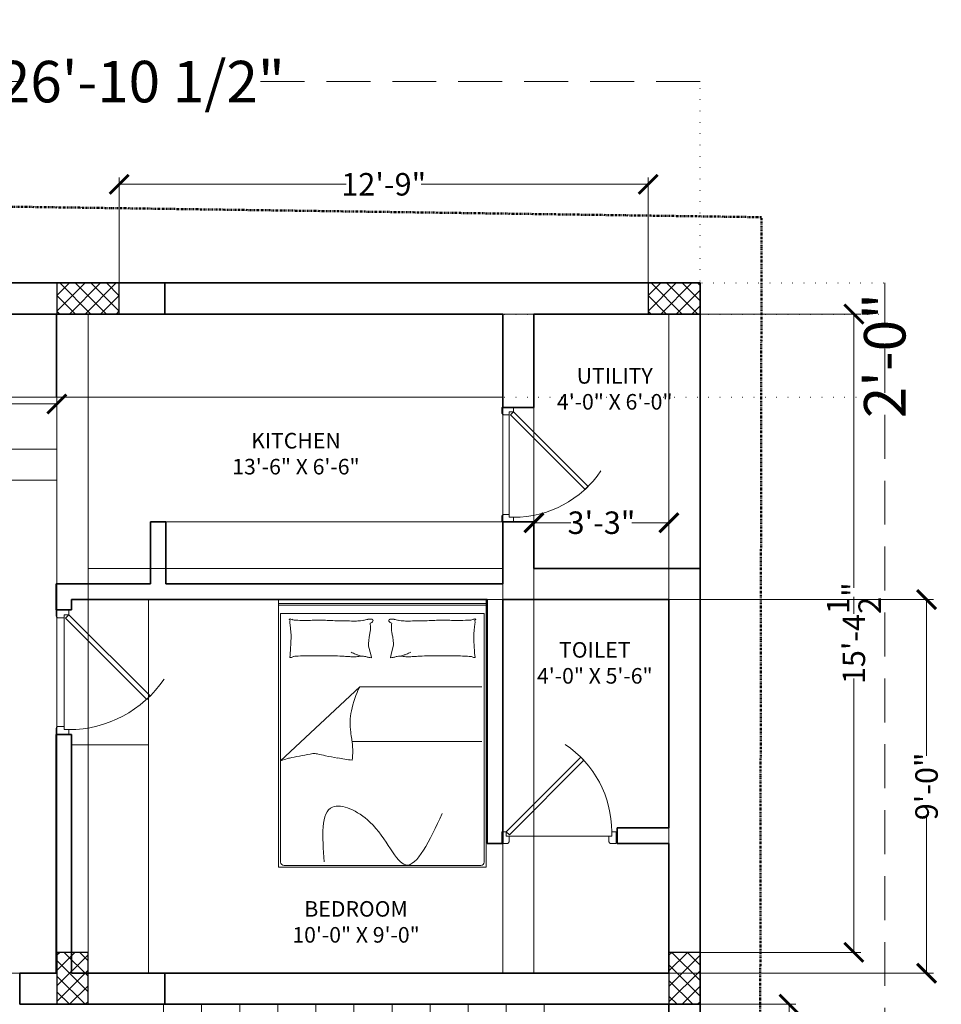
# Model space of a CAD drawing. Units: inches. Extents: x -16911 to -9621, y -48626 to -46270.
# Tile 14 of 20: x -11935 to -11669, y -46595 to -46311. Entities that reach past the tile are written whole.
import ezdxf

# ---------------------------------------------------------------- set-up
doc = ezdxf.new("R2010")
doc.units = ezdxf.units.IN
for name, pattern in [('DASHDOT', [1, 0.5, -0.25, 0, -0.25]), ('DASHED', [19.05, 12.7, -6.35]), ('DOT2', [3.175, 0, -3.175])]:
    doc.linetypes.add(name, pattern=pattern)
for name, color, linetype, lineweight in [('A-ANNO-DIMS', 2, 'Continuous', 13), ('A-AREA-IDEN', 3, 'Continuous', 18), ('A-DOOR', 4, 'Continuous', 18), ('A-FLOR-STRS', 3, 'Continuous', 18), ('A-FURN', 8, 'Continuous', 13), ('A-WALL', 7, 'Continuous', 35), ('C-PROP', 6, 'DASHDOT', 50), ('column', 12, 'Continuous', 30), ('DOOR', 143, 'Continuous', 9), ('EXT BEAM', 132, 'Continuous', 13), ('furniture', 35, 'Continuous', 15), ('S-BEAM', 132, 'Continuous', 25), ('S-COLS', 1, 'Continuous', 30)]:
    doc.layers.add(name, color=color, linetype=linetype, lineweight=lineweight)
doc.styles.add('style3', font='times.ttf')
doc.styles.add('style9', font='swisscl.ttf', dxfattribs={"height": 12})
doc.dimstyles.new('Dim9', dxfattribs={"dimtxt": 10, "dimasz": 0.199219, "dimexe": 1, "dimexo": 0.5, "dimgap": 1, "dimtad": 0, "dimdec": 1, "dimzin": 0, "dimdsep": 46, "dimlunit": 4, "dimtxsty": 'style9', "dimblk": 'ARCHTICK', "dimcen": 0.09, "dimclrd": 256, "dimclrt": 256, "dimadec": 0, "dimazin": 0, "dimtfac": 1, "dimtdec": 1, "dimtix": 1, "dimtofl": 0, "dimtmove": 1, "dimatfit": 3, "dimfxl": 9, "dimtolj": 1, "dimtzin": 0, "dimlwd": -1, "dimarcsym": 0})
doc.dimstyles.new('S.S.S', dxfattribs={"dimtxt": 6.5, "dimasz": 5.5, "dimexe": 2, "dimexo": 0, "dimgap": 0.09, "dimtad": 0, "dimdec": 1, "dimzin": 3, "dimdsep": 46, "dimlunit": 4, "dimtxsty": 'style3', "dimblk": 'ARCHTICK', "dimcen": 2.5, "dimclrd": 252, "dimclre": 256, "dimclrt": 7, "dimadec": 0, "dimazin": 0, "dimtfac": 1, "dimtdec": 1, "dimtix": 1, "dimtofl": 0, "dimtmove": 0, "dimatfit": 3, "dimfxl": 2, "dimtolj": 1, "dimtzin": 0, "dimlwd": 13, "dimlwe": 15, "dimarcsym": 0})

# ---------------------------------------------------------------- blocks, each defined once
blk = doc.blocks.new('hjuyuiuyk')
at = {"layer": 'furniture'}
for p, q in [((-19327.49, -39738.98), (-19327.49, -39737.31)), ((-19327.49, -39737.31), (-19267.49, -39737.31, 0)), ((-19327.49, -39746.54), (-19327.49, -39737.31)), ((-19267.49, -39738.5), (-19327.49, -39738.5, 0)), ((-19327.49, -39738.5, 0), (-19327.49, -39814.72, 0)), ((-19327.49, -39738.5), (-19327.49, -39814.72)), ((-19267.49, -39738.5, 0), (-19327.49, -39738.5)), ((-19267.49, -39738.98, 0), (-19327.49, -39738.98)), ((-19267.49, -39737.31, 0), (-19267.49, -39738.98, 0)), ((-19267.49, -39746.54, 0), (-19267.49, -39737.31, 0)), ((-19267.49, -39814.72), (-19267.49, -39738.5)), ((-19267.49, -39814.72, 0), (-19267.49, -39738.5, 0)), ((-19268.1, -39741.33), (-19326.9, -39741.33)), ((-19326.9, -39741.33), (-19326.9, -39813.21)), ((-19268.1, -39813.21), (-19268.1, -39741.33)), ((-19300.88, -39753.22, 0), (-19301.49, -39750.81, 0)), ((-19294.97, -39753.22, 0), (-19294.37, -39750.81, 0)), ((-19300.67, -39754.09, 0), (-19300.88, -39753.22, 0)), ((-19295.19, -39754.09, 0), (-19294.97, -39753.22, 0)), ((-19304.07, -39762.52), (-19326.9, -39783.91)), ((-19304.07, -39762.52), (-19268.82, -39762.52)), ((-19268.82, -39778.34), (-19306.29, -39778.34)), ((-19326.9, -39813.21), (-19326.9, -39783.91)), ((-19327.49, -39814.72, 0), (-19267.49, -39814.72)), ((-19327.49, -39814.72), (-19267.49, -39814.72, 0)), ((-19269.1, -39814.21), (-19325.9, -39814.21)), ((-19325.9, -39814.21), (-19269.1, -39814.21))]:
    blk.add_line(p, q, dxfattribs=at)
for centre, radius, start, end in [((-19324.36, -39743.07, 0), 0.0997, 111.7883, 160.436), ((-19324.39, -39743.06, 0), 0.0676, 160.436, 281.8931), ((-19324.12, -39743.66, 0), 0.732, 94.3025, 111.7883), ((-19324.35, -39743.25, 0), 0.125, 21.9904, 101.8931), ((-19323.34, -39743.89, 0), 0.956, 158.579, 188.1335), ((-19317.18, -39743.01, 0), 7.17, 188.1335, 192.1095), ((-19324.65, -39743.37, 0), 0.455, 338.579, 21.9904), ((-19329.85, -39745.73, 0), 5.78, 7.6809, 12.1095), ((-19324.11, -39743.77, 0), 0.842, 59.3487, 94.3025), ((-19350.51, -39748.51, 0), 26.62, 3.3687, 7.6809), ((-19322.88, -39741.69, 0), 1.57, 239.3487, 264.7408), ((-19319.6, -39692.5, 0), 50.87, 266.1399, 268.6002), ((-19319.84, -39713.09, 0), 30.28, 268.0921, 271.2808), ((-19320.24, -39695.07, 0), 48.31, 271.2808, 273.4034), ((-19316.15, -39763.89, 0), 20.63, 90.1553, 93.4034), ((-19316.09, -39783.15, 0), 39.89, 86.9902, 90.1553), ((-19305.86, -39588.51, 0), 155.02, 266.9902, 268.5957), ((-19305.42, -39570.46, 0), 173.07, 268.5957, 270), ((-19305.42, -39718.38, 0), 25.15, 270, 273.6841), ((-19304.03, -39739.9, 0), 3.58, 273.6841, 287.1951), ((-19300.46, -39751.46, 0), 8.51, 98.4372, 107.1951), ((-19301.02, -39747.69, 0), 4.7, 90, 98.4372), ((-19301.12, -39743.14, 0), 0.997, 274.4002, 333.4195), ((-19315.3, -39745.68, 0), 14.34, 360, 6.2324), ((-19306.91, -39745.68, 0), 5.95, 350.3156, 360), ((-19301.02, -39745.63, 0), 2.64, 78.7276, 90), ((-19300.58, -39743.42, 0), 0.383, 333.4195, 78.7276), ((-19295.28, -39743.42, 0), 0.383, 101.2724, 206.5805), ((-19294.73, -39743.14, 0), 0.997, 206.5805, 265.5998), ((-19294.84, -39745.63, 0), 2.64, 90, 101.2724), ((-19280.55, -39745.68, 0), 14.34, 173.7676, 180), ((-19288.94, -39745.68, 0), 5.95, 180, 189.6844), ((-19294.84, -39747.69, 0), 4.7, 81.5628, 90), ((-19295.39, -39751.46, 0), 8.51, 72.8049, 81.5628), ((-19291.82, -39739.9, 0), 3.58, 252.8049, 266.3159), ((-19290.43, -39718.38, 0), 25.15, 266.3159, 270), ((-19290.43, -39570.46, 0), 173.07, 270, 271.4043), ((-19289.99, -39588.51, 0), 155.02, 271.4043, 273.0098), ((-19279.76, -39783.15, 0), 39.89, 89.8447, 93.0098), ((-19279.7, -39763.89, 0), 20.63, 86.5966, 89.8447), ((-19275.61, -39695.07, 0), 48.31, 266.5966, 268.7192), ((-19276.02, -39713.09, 0), 30.28, 268.7192, 271.9079), ((-19276.73, -39645.13, 0), 98.25, 271.0069, 272.7772), ((-19272.12, -39741.69, 0), 1.57, 275.2592, 300.6513), ((-19270.89, -39743.77, 0), 0.842, 85.6975, 120.6513), ((-19244.49, -39748.51, 0), 26.62, 172.3191, 176.6313), ((-19265.15, -39745.73, 0), 5.78, 167.8905, 172.3191), ((-19270.88, -39743.66, 0), 0.732, 68.2117, 85.6975), ((-19270.35, -39743.37, 0), 0.455, 158.0096, 201.421), ((-19277.82, -39743.01, 0), 7.17, 347.8905, 351.8665), ((-19270.65, -39743.25, 0), 0.125, 78.1069, 158.0096), ((-19271.66, -39743.89, 0), 0.956, 351.8665, 21.421), ((-19270.61, -39743.06, 0), 0.0676, 258.1069, 19.564), ((-19270.64, -39743.07, 0), 0.0997, 19.564, 68.2117), ((-19343.69, -39748.11, 0), 19.79, 358.3669, 3.3687), ((-19282.35, -39751.13, 0), 19.21, 171.9949, 177.3351), ((-19292.22, -39749.75, 0), 9.25, 167.8016, 171.9949), ((-19326.4, -39742.36, 0), 25.72, 347.8016, 350.3156), ((-19269.45, -39742.36, 0), 25.72, 189.6844, 192.1984), ((-19303.63, -39749.75, 0), 9.25, 8.0051, 12.1984), ((-19313.5, -39751.13, 0), 19.21, 2.6649, 8.0051), ((-19251.31, -39748.11, 0), 19.79, 176.6313, 181.6331), ((-19720.99, -39728.47, 0), 397.61, 356.4951, 356.945), ((-19363.7, -39747.54, 0), 39.81, 356.945, 358.3669), ((-19299.57, -39750.33, 0), 1.97, 177.3351, 194.0452), ((-19296.28, -39750.33, 0), 1.97, 345.9548, 2.6649), ((-19231.3, -39747.54, 0), 39.81, 181.6331, 183.055), ((-18874.01, -39728.47, 0), 397.61, 183.055, 183.5049), ((-19323.69, -39753.93, 0), 0.564, 170.0016, 196.6978), ((-19333.47, -39752.21, 0), 9.37, 350.0016, 356.4951), ((-19324.19, -39754.08, 0), 0.0385, 196.6978, 277.1204), ((-19324.51, -39751.59, 0), 2.55, 277.1204, 286.2212), ((-19324.42, -39751.9, 0), 2.23, 286.2212, 297.4439), ((-19322.81, -39754.99, 0), 1.25, 102.448, 117.4439), ((-19322.32, -39757.22, 0), 3.54, 93.574, 102.448), ((-19318.44, -39837.61, 0), 84.03, 90.9755, 92.7955), ((-19315.55, -39952.16, 0), 198.61, 89.4461, 91.2473), ((-19314.9, -39885.06, 0), 131.51, 87.2326, 89.4461), ((-19310.57, -39795.48, 0), 41.81, 85.4012, 87.2326), ((-19304.32, -39717.78, 0), 36.14, 265.4012, 267.3712), ((-19297.32, -39733.09, 0), 21.54, 244.6889, 246.5156), ((-19305.66, -39747.05, 0), 6.83, 267.3712, 281.4827), ((-19297.32, -39733.09, 0), 21.54, 246.5156, 248.3423), ((-19297.32, -39733.09, 0), 21.54, 248.3423, 250.572), ((-19297.32, -39733.09, 0), 21.54, 250.572, 252.8018), ((-19303.46, -39757.91, 0), 4.25, 83.5659, 101.4827), ((-19303.37, -39757.16, 0), 3.49, 72.6136, 83.5659), ((-19300.33, -39747.43, 0), 6.7, 252.6136, 260.5159), ((-19300.13, -39746.25, 0), 7.9, 260.5159, 265.9171), ((-19300.69, -39754.1, 0), 0.0267, 265.9171, 14.0449), ((-19295.16, -39754.1, 0), 0.0267, 165.9551, 274.0829), ((-19295.72, -39746.25, 0), 7.9, 274.0829, 279.4841), ((-19295.52, -39747.43, 0), 6.7, 279.4841, 287.3864), ((-19292.48, -39757.16, 0), 3.49, 96.4341, 107.3864), ((-19292.39, -39757.91, 0), 4.25, 78.5173, 96.4341), ((-19298.54, -39733.09, 0), 21.54, 287.1982, 289.428), ((-19290.19, -39747.05, 0), 6.83, 258.5173, 272.6288), ((-19298.54, -39733.09, 0), 21.54, 289.428, 291.6577), ((-19298.54, -39733.09, 0), 21.54, 291.6577, 293.4844), ((-19298.54, -39733.09, 0), 21.54, 293.4844, 295.3111), ((-19291.53, -39717.78, 0), 36.14, 272.6288, 274.5988), ((-19285.28, -39795.48, 0), 41.81, 92.7674, 94.5988), ((-19280.95, -39885.06, 0), 131.51, 90.5539, 92.7674), ((-19280.3, -39952.16, 0), 198.61, 88.7527, 90.5539), ((-19277.1, -39805.01, 0), 51.42, 86.426, 88.7527), ((-19274.68, -39799.75, 0), 46.07, 86.5575, 89.0171), ((-19272.19, -39754.99, 0), 1.25, 62.5561, 77.552), ((-19270.58, -39751.9, 0), 2.23, 242.5561, 253.7788), ((-19270.49, -39751.59, 0), 2.55, 253.7788, 262.8796), ((-19261.53, -39752.21, 0), 9.37, 183.5049, 189.9984), ((-19270.81, -39754.08, 0), 0.0385, 262.8796, 343.3022), ((-19271.31, -39753.93, 0), 0.564, 343.3022, 9.9984), ((-19279.47, -39774.89), 27.53, 153.3084, 168.7423), ((-19287.94, -39773.2), 18.89, 168.7423, 187.3994), ((-19242.78, -39767.34), 64.43, 187.3994, 189.2719), ((-19333.07, -39782.08), 27.05, 6.3817, 9.2719), ((-19321.79, -39780.82), 15.7, 359.2313, 6.3817), ((-19287.64, -39956.87), 177.57, 99.7243, 101.7196), ((-19317.24, -39783.9), 2.09, 82.2696, 100.7276), ((-19317.9, -39788.76), 6.99, 76.8096, 82.2696), ((-19295.64, -39693.77), 90.57, 256.8096, 258.3259), ((-19295.11, -39691.23), 93.17, 258.3259, 260.505), ((-19336.71, -39780.62), 30.63, 354.1141, 359.2313), ((-19306.77, -39846.83), 66.07, 105.9352, 107.7364), ((-19318.41, -39806.06), 23.67, 102.9255, 105.9352), ((-19288.03, -39648.9), 136.08, 260.505, 262.308), ((-19325.9, -39813.21), 1, 180, 270), ((-19269.1, -39813.21), 1, 270, 0)]:
    blk.add_arc(centre, radius, start, end, dxfattribs=at)
blk.add_open_spline([(-19280.24, -39799.21), (-19283.87, -39806.94), (-19290.73, -39821.55), (-19298.08, -39801.09), (-19315.85, -39793.47), (-19314.86, -39805.92), (-19314.29, -39813.13)], degree=3, knots=[0, 0, 0, 0, 18.167809, 34.338432, 45.972904, 61.997799, 61.997799, 61.997799, 61.997799], dxfattribs=at)
blk = doc.blocks.new('A$C1C9D3E54')
at = {"layer": 'DOOR'}
blk.add_line((18676.53, 5780.72), (18710.53, 5780.72), dxfattribs=at)
blk.add_lwpolyline([(18685.01, 5806.62), (18710.47, 5781.16), (18711.53, 5782.22), (18686.07, 5807.68), (18685.01, 5806.62)], dxfattribs=at)
blk.add_lwpolyline([(18674.03, 5778.22), (18676.03, 5778.22), (18674.03, 5778.22), (18674.03, 5782.22), (18675.53, 5782.22), (18675.53, 5780.72), (18676.53, 5780.72), (18676.53, 5778.72), (18676.41, 5778.72), (18676.41, 5778.6, -0.414214), (18676.16, 5778.35), (18676.03, 5778.35), (18676.03, 5778.22)], format="xyb", dxfattribs=at)
blk.add_lwpolyline([(18713.03, 5782.22), (18711.53, 5782.22), (18711.53, 5780.72), (18710.53, 5780.72), (18710.53, 5778.72), (18710.66, 5778.72), (18710.66, 5778.6, 0.414214), (18710.91, 5778.35), (18711.03, 5778.35), (18711.03, 5778.22), (18713.03, 5778.22), (18711.03, 5778.22), (18713.03, 5778.22), (18713.03, 5782.22)], format="xyb", close=True, dxfattribs=at)
blk.add_arc((18711.53, 5782.22), 36, 124.0336, 180, dxfattribs=at)
blk = doc.blocks.new('COLUMNS')
at = {"layer": 'column'}
h = blk.add_hatch(dxfattribs=at)
h.set_pattern_fill('ANSI37', color=256, angle=-810)
h.set_pattern_definition([(315, (-70004.5392, -80151.7886), (2.24506403, 2.24506403), []), (45, (-70004.5392, -80151.7886), (-2.24506403, 2.24506403), [])])
h.paths.add_polyline_path([(-11924.72, -46386.86), (-11924.72, -46395.86), (-11906.72, -46395.86), (-11906.72, -46386.86)])
h = blk.add_hatch(dxfattribs=at)
h.set_pattern_fill('ANSI37', color=256, angle=-810)
h.set_pattern_definition([(315, (-69833.7395, -80151.7886), (2.24506403, 2.24506403), []), (45, (-69833.7395, -80151.7886), (-2.24506403, 2.24506403), [])])
h.paths.add_polyline_path([(-11753.92, -46386.86), (-11753.92, -46395.86), (-11738.92, -46395.86), (-11738.92, -46386.86)])
h = blk.add_hatch(dxfattribs=at)
h.set_pattern_fill('ANSI37', color=256, angle=-720)
h.set_pattern_definition([(45, (21840.2088, -104675.1704), (-2.24506403, 2.24506403), []), (135, (21840.2088, -104675.1704), (-2.24506403, -2.24506403), [])])
h.paths.add_polyline_path([(-11924.72, -46595.36), (-11915.72, -46595.36), (-11915.72, -46580.36), (-11924.72, -46580.36)])
h = blk.add_hatch(dxfattribs=at)
h.set_pattern_fill('ANSI37', color=256, angle=-900)
h.set_pattern_definition([(225, (-45503.8578, 11499.4594), (2.24506403, -2.24506403), []), (315, (-45503.8578, 11499.4594), (2.24506403, 2.24506403), [])])
h.paths.add_polyline_path([(-11738.92, -46580.36), (-11747.92, -46580.36), (-11747.92, -46595.36), (-11738.92, -46595.36)])
at = {"layer": 'column', "ltscale": 0.05}
for points in [[(-11906.72, -46395.86), (-11906.72, -46386.86), (-11924.72, -46386.86), (-11924.72, -46395.86)], [(-11738.92, -46395.86), (-11738.92, -46386.86), (-11753.92, -46386.86), (-11753.92, -46395.86)], [(-11915.72, -46580.36), (-11924.72, -46580.36), (-11924.72, -46595.36), (-11915.72, -46595.36)], [(-11747.92, -46595.36), (-11738.92, -46595.36), (-11738.92, -46580.36), (-11747.92, -46580.36)]]:
    blk.add_lwpolyline(points, close=True, dxfattribs=at)
blk = doc.blocks.new('TYPICAL BEAMS G-2')
at = {"layer": 'EXT BEAM'}
for p, q in [((-12061.47, -47658.74), (-11738.92, -47658.74)), ((-11738.92, -48216.7), (-11738.92, -47658.74)), ((-12052.47, -47667.74), (-11924.72, -47667.74)), ((-11924.72, -47667.74), (-11924.72, -47858.24)), ((-11915.72, -47667.74), (-11747.92, -47667.74)), ((-11915.72, -47667.74), (-11915.72, -47858.24)), ((-11795.92, -47667.74), (-11795.92, -47858.24)), ((-11786.92, -47667.74), (-11786.92, -47858.24)), ((-11747.92, -47858.24), (-11747.92, -47667.74)), ((-12052.47, -47706.74), (-11924.72, -47706.74)), ((-12052.47, -47715.74), (-11924.72, -47715.74)), ((-11915.72, -47741.24), (-11795.92, -47741.24)), ((-11786.92, -47741.24), (-11747.92, -47741.24)), ((-11915.72, -47750.24), (-11795.92, -47750.24)), ((-11786.92, -47750.24), (-11747.92, -47750.24)), ((-12052.47, -47858.24), (-11924.72, -47858.24)), ((-11915.72, -47858.24), (-11747.92, -47858.24)), ((-11915.72, -47867.24), (-11747.92, -47867.24))]:
    blk.add_line(p, q, dxfattribs=at)
blk = doc.blocks.new('_ArchTick')
at = {"color": 0, "linetype": 'ByBlock', "const_width": 0.15}
blk.add_lwpolyline([(-0.5, -0.5), (0.5, 0.5)], dxfattribs=at)
blk = doc.blocks.new('*D30')
at = {"layer": 'A-ANNO-DIMS', "color": 0, "lineweight": 15, "transparency": 16777216}
for p, q in [((-11738.92, -46395.86), (-11692.5, -46395.86)), ((-11738.92, -46580.36), (-11692.5, -46580.36))]:
    blk.add_line(p, q, dxfattribs=at)
at = {"layer": 'A-ANNO-DIMS', "color": 0, "lineweight": 13, "transparency": 16777216}
for p, q in [((-11694.5, -46395.86), (-11694.5, -46475.01)), ((-11694.5, -46580.36), (-11694.5, -46501.2))]:
    blk.add_line(p, q, dxfattribs=at)
at = {"layer": 'Defpoints', "color": 0, "transparency": 16777216}
for p in [(-11738.92, -46395.86), (-11738.92, -46580.36), (-11694.5, -46580.36)]:
    blk.add_point(p, dxfattribs=at)
at = {"layer": 'A-ANNO-DIMS', "color": 0, "lineweight": 13, "transparency": 16777216, "xscale": 5.5, "yscale": 5.5, "zscale": 5.5}
for p, rotation in [((-11694.5, -46395.86), 90), ((-11694.5, -46580.36), 270)]:
    blk.add_blockref('_ArchTick', p, dxfattribs=dict(at, rotation=rotation))
at = {"layer": 'A-ANNO-DIMS', "color": 0, "transparency": 16777216, "insert": (-11694.5, -46488.11), "char_height": 6.5, "attachment_point": 5, "rotation": 90, "style": 'style3'}
blk.add_mtext('\\A1;15\'-4{\\H1x;\\S1/2;}"', dxfattribs=at)
blk = doc.blocks.new('*D31')
at = {"layer": 'A-ANNO-DIMS', "color": 0, "lineweight": 15, "transparency": 16777216}
for p, q in [((-11906.72, -46386.86), (-11906.72, -46356.34)), ((-11753.92, -46386.86), (-11753.92, -46356.34))]:
    blk.add_line(p, q, dxfattribs=at)
at = {"layer": 'A-ANNO-DIMS', "color": 0, "lineweight": 13, "transparency": 16777216}
for p, q in [((-11906.72, -46358.34), (-11841.15, -46358.34)), ((-11753.92, -46358.34), (-11819.5, -46358.34))]:
    blk.add_line(p, q, dxfattribs=at)
at = {"layer": 'Defpoints', "color": 0, "transparency": 16777216}
for p in [(-11906.72, -46358.34), (-11906.72, -46386.86), (-11753.92, -46386.86)]:
    blk.add_point(p, dxfattribs=at)
at = {"layer": 'A-ANNO-DIMS', "color": 0, "lineweight": 13, "transparency": 16777216, "xscale": 5.5, "yscale": 5.5, "zscale": 5.5, "rotation": 180}
blk.add_blockref('_ArchTick', (-11906.72, -46358.34), dxfattribs=at)
at = {"layer": 'A-ANNO-DIMS', "color": 0, "lineweight": 13, "transparency": 16777216, "xscale": 5.5, "yscale": 5.5, "zscale": 5.5}
blk.add_blockref('_ArchTick', (-11753.92, -46358.34), dxfattribs=at)
at = {"layer": 'A-ANNO-DIMS', "color": 0, "transparency": 16777216, "insert": (-11830.32, -46358.34), "char_height": 6.5, "attachment_point": 5, "style": 'style3'}
blk.add_mtext('\\A1;12\'-9"', dxfattribs=at)
blk = doc.blocks.new('*D32')
at = {"layer": 'A-ANNO-DIMS', "color": 0, "lineweight": 15, "transparency": 16777216}
for p, q in [((-11747.92, -46595.36), (-11711.23, -46595.36)), ((-11746.42, -46667.36), (-11711.23, -46667.36))]:
    blk.add_line(p, q, dxfattribs=at)
at = {"layer": 'A-ANNO-DIMS', "color": 0, "lineweight": 13, "transparency": 16777216}
for p, q in [((-11713.23, -46595.36), (-11713.23, -46622.57)), ((-11713.23, -46667.36), (-11713.23, -46640.14))]:
    blk.add_line(p, q, dxfattribs=at)
at = {"layer": 'Defpoints', "color": 0, "transparency": 16777216}
for p in [(-11747.92, -46595.36), (-11713.23, -46595.36), (-11746.42, -46667.36)]:
    blk.add_point(p, dxfattribs=at)
at = {"layer": 'A-ANNO-DIMS', "color": 0, "lineweight": 13, "transparency": 16777216, "xscale": 5.5, "yscale": 5.5, "zscale": 5.5}
for p, rotation in [((-11713.23, -46595.36), 90), ((-11713.23, -46667.36), 270)]:
    blk.add_blockref('_ArchTick', p, dxfattribs=dict(at, rotation=rotation))
at = {"layer": 'A-ANNO-DIMS', "color": 0, "transparency": 16777216, "insert": (-11713.23, -46631.36), "char_height": 6.5, "attachment_point": 5, "rotation": 90, "style": 'style3'}
blk.add_mtext('\\A1;6\'-0"', dxfattribs=at)
blk = doc.blocks.new('*D45')
at = {"layer": 'A-ANNO-DIMS', "color": 0, "lineweight": 15, "transparency": 16777216}
for p, q in [((-12052.47, -46434.86), (-12052.47, -46419.84)), ((-11924.72, -46434.86), (-11924.72, -46419.84))]:
    blk.add_line(p, q, dxfattribs=at)
at = {"layer": 'A-ANNO-DIMS', "color": 0, "lineweight": 13, "transparency": 16777216}
for p, q in [((-12052.47, -46421.84), (-11999.43, -46421.84)), ((-11924.72, -46421.84), (-11977.77, -46421.84))]:
    blk.add_line(p, q, dxfattribs=at)
at = {"layer": 'Defpoints', "color": 0, "transparency": 16777216}
for p in [(-11924.72, -46421.84), (-12052.47, -46434.86), (-11924.72, -46434.86)]:
    blk.add_point(p, dxfattribs=at)
at = {"layer": 'A-ANNO-DIMS', "color": 0, "lineweight": 13, "transparency": 16777216, "xscale": 5.5, "yscale": 5.5, "zscale": 5.5, "rotation": 180}
blk.add_blockref('_ArchTick', (-12052.47, -46421.84), dxfattribs=at)
at = {"layer": 'A-ANNO-DIMS', "color": 0, "lineweight": 13, "transparency": 16777216, "xscale": 5.5, "yscale": 5.5, "zscale": 5.5}
blk.add_blockref('_ArchTick', (-11924.72, -46421.84), dxfattribs=at)
at = {"layer": 'A-ANNO-DIMS', "color": 0, "transparency": 16777216, "insert": (-11988.6, -46421.84), "char_height": 6.5, "attachment_point": 5, "style": 'style3'}
blk.add_mtext('\\A1;10\'-8"', dxfattribs=at)
blk = doc.blocks.new('*D46')
at = {"layer": 'A-ANNO-DIMS', "color": 0, "lineweight": 15, "transparency": 16777216}
for p, q in [((-11786.92, -46478.36), (-11786.92, -46454.16)), ((-11747.92, -46478.36), (-11747.92, -46454.16))]:
    blk.add_line(p, q, dxfattribs=at)
at = {"layer": 'A-ANNO-DIMS', "color": 0, "lineweight": 13, "transparency": 16777216}
for p, q in [((-11786.92, -46456.16), (-11776.22, -46456.16)), ((-11747.92, -46456.16), (-11758.63, -46456.16))]:
    blk.add_line(p, q, dxfattribs=at)
at = {"layer": 'Defpoints', "color": 0, "transparency": 16777216}
for p in [(-11747.92, -46456.16), (-11786.92, -46478.36), (-11747.92, -46478.36)]:
    blk.add_point(p, dxfattribs=at)
at = {"layer": 'A-ANNO-DIMS', "color": 0, "lineweight": 13, "transparency": 16777216, "xscale": 5.5, "yscale": 5.5, "zscale": 5.5, "rotation": 180}
blk.add_blockref('_ArchTick', (-11786.92, -46456.16), dxfattribs=at)
at = {"layer": 'A-ANNO-DIMS', "color": 0, "lineweight": 13, "transparency": 16777216, "xscale": 5.5, "yscale": 5.5, "zscale": 5.5}
blk.add_blockref('_ArchTick', (-11747.92, -46456.16), dxfattribs=at)
at = {"layer": 'A-ANNO-DIMS', "color": 0, "transparency": 16777216, "insert": (-11767.42, -46456.16), "char_height": 6.5, "attachment_point": 5, "style": 'style3'}
blk.add_mtext('\\A1;3\'-3"', dxfattribs=at)
blk = doc.blocks.new('*D47')
at = {"layer": 'A-ANNO-DIMS', "color": 0, "lineweight": 15, "transparency": 16777216}
for p, q in [((-11747.92, -46478.36), (-11671.51, -46478.36)), ((-11753.13, -46586.36), (-11671.51, -46586.36))]:
    blk.add_line(p, q, dxfattribs=at)
at = {"layer": 'A-ANNO-DIMS', "color": 0, "lineweight": 13, "transparency": 16777216}
for p, q in [((-11673.51, -46478.36), (-11673.51, -46523.55)), ((-11673.51, -46586.36), (-11673.51, -46541.16))]:
    blk.add_line(p, q, dxfattribs=at)
at = {"layer": 'Defpoints', "color": 0, "transparency": 16777216}
for p in [(-11747.92, -46478.36), (-11753.13, -46586.36), (-11673.51, -46586.36)]:
    blk.add_point(p, dxfattribs=at)
at = {"layer": 'A-ANNO-DIMS', "color": 0, "lineweight": 13, "transparency": 16777216, "xscale": 5.5, "yscale": 5.5, "zscale": 5.5}
for p, rotation in [((-11673.51, -46478.36), 90), ((-11673.51, -46586.36), 270)]:
    blk.add_blockref('_ArchTick', p, dxfattribs=dict(at, rotation=rotation))
at = {"layer": 'A-ANNO-DIMS', "color": 0, "transparency": 16777216, "insert": (-11673.51, -46532.36), "char_height": 6.5, "attachment_point": 5, "rotation": 90, "style": 'style3'}
blk.add_mtext('\\A1;9\'-0"', dxfattribs=at)
blk = doc.blocks.new('*D114')
at = {"layer": 'A-ANNO-DIMS', "color": 0, "linetype": 'DOT2', "lineweight": -2, "transparency": 16777216}
for p, q in [((-12061.47, -46386.36), (-12061.47, -46327.66)), ((-11738.92, -46386.36), (-11738.92, -46327.66))]:
    blk.add_line(p, q, dxfattribs=at)
at = {"layer": 'A-ANNO-DIMS', "linetype": 'DASHED', "transparency": 16777216}
for p, q in [((-12061.47, -46328.66), (-11933.21, -46328.66)), ((-11738.92, -46328.66), (-11867.19, -46328.66))]:
    blk.add_line(p, q, dxfattribs=at)
at = {"layer": 'Defpoints', "color": 0, "transparency": 16777216}
for p in [(-11738.92, -46328.66), (-12061.47, -46386.86), (-11738.92, -46386.86)]:
    blk.add_point(p, dxfattribs=at)
at = {"layer": 'A-ANNO-DIMS', "transparency": 16777216, "xscale": 0.19921875, "yscale": 0.19921875, "zscale": 0.19921875, "rotation": 180}
blk.add_blockref('_ArchTick', (-12061.47, -46328.66), dxfattribs=at)
at = {"layer": 'A-ANNO-DIMS', "transparency": 16777216, "xscale": 0.19921875, "yscale": 0.19921875, "zscale": 0.19921875}
blk.add_blockref('_ArchTick', (-11738.92, -46328.66), dxfattribs=at)
at = {"layer": 'A-ANNO-DIMS', "transparency": 16777216, "insert": (-11900.2, -46328.66), "char_height": 12, "attachment_point": 5, "style": 'style9'}
blk.add_mtext('\\A1;26\'-10 1/2"', dxfattribs=at)
blk = doc.blocks.new('*D115')
at = {"layer": 'A-ANNO-DIMS', "color": 0, "linetype": 'DOT2', "lineweight": -2, "transparency": 16777216}
for p, q in [((-11738.42, -46386.86), (-11684.58, -46386.86)), ((-11738.42, -46944.81), (-11684.58, -46944.81))]:
    blk.add_line(p, q, dxfattribs=at)
at = {"layer": 'A-ANNO-DIMS', "linetype": 'DASHED', "transparency": 16777216}
for p, q in [((-11685.58, -46386.86), (-11685.58, -46648.2)), ((-11685.58, -46944.81), (-11685.58, -46683.47))]:
    blk.add_line(p, q, dxfattribs=at)
at = {"layer": 'Defpoints', "color": 0, "transparency": 16777216}
for p in [(-11738.92, -46386.86), (-11738.92, -46944.81), (-11685.58, -46944.81)]:
    blk.add_point(p, dxfattribs=at)
at = {"layer": 'A-ANNO-DIMS', "transparency": 16777216, "xscale": 0.19921875, "yscale": 0.19921875, "zscale": 0.19921875}
for p, rotation in [((-11685.58, -46386.86), 90), ((-11685.58, -46944.81), 270)]:
    blk.add_blockref('_ArchTick', p, dxfattribs=dict(at, rotation=rotation))
at = {"layer": 'A-ANNO-DIMS', "transparency": 16777216, "insert": (-11685.58, -46665.83), "char_height": 12, "attachment_point": 5, "rotation": 90, "style": 'style9'}
blk.add_mtext('\\A1;46\'-6"', dxfattribs=at)
blk = doc.blocks.new('*D116')
at = {"layer": 'A-ANNO-DIMS', "color": 0, "linetype": 'DOT2', "lineweight": -2, "transparency": 16777216}
for p, q in [((-11795.42, -46395.86), (-11684.58, -46395.86)), ((-11795.42, -46419.86), (-11684.58, -46419.86))]:
    blk.add_line(p, q, dxfattribs=at)
at = {"layer": 'A-ANNO-DIMS', "linetype": 'DASHED', "transparency": 16777216}
for p, q in [((-11685.58, -46395.86), (-11685.58, -46395.66)), ((-11685.58, -46419.86), (-11685.58, -46420.05))]:
    blk.add_line(p, q, dxfattribs=at)
at = {"layer": 'Defpoints', "color": 0, "transparency": 16777216}
for p in [(-11795.92, -46395.86), (-11795.92, -46419.86), (-11685.58, -46419.86)]:
    blk.add_point(p, dxfattribs=at)
at = {"layer": 'A-ANNO-DIMS', "transparency": 16777216, "xscale": 0.19921875, "yscale": 0.19921875, "zscale": 0.19921875}
for p, rotation in [((-11685.58, -46395.86), 270), ((-11685.58, -46419.86), 90)]:
    blk.add_blockref('_ArchTick', p, dxfattribs=dict(at, rotation=rotation))
at = {"layer": 'A-ANNO-DIMS', "transparency": 16777216, "insert": (-11685.58, -46407.86), "char_height": 12, "attachment_point": 5, "rotation": 90, "style": 'style9'}
blk.add_mtext('\\A1;2\'-0"', dxfattribs=at)

msp = doc.modelspace()

# ---------------------------------------------------------------- linework, layer by layer
at = {"layer": 'A-FLOR-STRS', "ltscale": 10}
for p, q in [((-11893.925, -46595.355), (-11893.925, -46667.355)), ((-11882.925, -46595.355), (-11882.925, -46667.355)), ((-11871.925, -46595.355), (-11871.925, -46667.355)), ((-11860.925, -46595.355), (-11860.925, -46667.355)), ((-11849.925, -46595.355), (-11849.925, -46667.355)), ((-11838.925, -46595.355), (-11838.925, -46667.355)), ((-11827.925, -46595.355), (-11827.925, -46667.355)), ((-11816.925, -46595.355), (-11816.925, -46667.355)), ((-11805.925, -46595.355), (-11805.925, -46667.355)), ((-11794.925, -46595.355), (-11794.925, -46667.355)), ((-11783.925, -46595.355), (-11783.925, -46667.355))]:
    msp.add_line(p, q, dxfattribs=at)
at = {"layer": 'A-FURN', "ltscale": 0.2}
for p, q in [((-11924.974, -46419.855), (-11924.974, -46395.855)), ((-11795.925, -46419.855), (-11959.474, -46419.855)), ((-11795.925, -46455.855), (-11893.224, -46455.855)), ((-11920.474, -46520.355), (-11898.224, -46520.355)), ((-11898.224, -46520.355), (-11898.224, -46586.355))]:
    msp.add_line(p, q, dxfattribs=at)
at = {"layer": 'A-FURN', "ltscale": 0.5}
msp.add_line((-11898.224, -46520.355), (-11898.224, -46478.355), dxfattribs=at)
at = {"layer": 'A-WALL'}
for p, q in [((-11738.925, -46386.855), (-11968.474, -46386.855)), ((-11893.506, -46386.855), (-11893.506, -46395.855)), ((-11738.925, -46386.855), (-11738.925, -46395.855)), ((-11795.925, -46395.855), (-11959.474, -46395.855)), ((-11795.925, -46395.855), (-11795.925, -46422.855)), ((-11738.925, -46395.855), (-11786.925, -46395.855)), ((-11786.925, -46395.855), (-11786.925, -46422.855)), ((-11738.925, -46395.855), (-11738.925, -46469.355)), ((-11795.925, -46422.855), (-11786.925, -46422.855)), ((-11897.724, -46473.855), (-11897.724, -46455.855)), ((-11893.224, -46455.855), (-11897.724, -46455.855)), ((-11893.224, -46473.855), (-11893.224, -46455.855)), ((-11795.925, -46455.855), (-11795.925, -46473.855)), ((-11795.925, -46455.855), (-11786.925, -46455.855)), ((-11786.925, -46455.855), (-11786.925, -46469.355)), ((-11738.925, -46469.355), (-11786.925, -46469.355)), ((-11738.925, -46469.355), (-11738.925, -46676.355)), ((-11924.974, -46481.355), (-11924.974, -46473.855)), ((-11897.724, -46473.855), (-11924.974, -46473.855)), ((-11795.925, -46473.855), (-11893.224, -46473.855)), ((-11920.474, -46481.355), (-11920.474, -46478.355)), ((-11800.425, -46478.355), (-11920.474, -46478.355)), ((-11800.425, -46478.355), (-11800.425, -46548.855)), ((-11747.925, -46478.355), (-11795.925, -46478.355)), ((-11795.925, -46478.355), (-11795.925, -46548.855)), ((-11747.925, -46478.355), (-11747.925, -46544.355)), ((-11924.974, -46481.355), (-11920.474, -46481.355)), ((-11924.974, -46586.355), (-11924.974, -46517.355)), ((-11924.974, -46517.355), (-11920.474, -46517.355)), ((-11920.474, -46586.355), (-11920.474, -46517.355)), ((-11747.925, -46544.355), (-11762.925, -46544.355)), ((-11762.925, -46544.355), (-11762.925, -46548.855)), ((-11795.925, -46548.855), (-11800.425, -46548.855)), ((-11747.925, -46548.855), (-11762.925, -46548.855)), ((-11747.925, -46548.855), (-11747.925, -46586.355)), ((-11924.974, -46586.355), (-11935.474, -46586.355)), ((-11935.474, -46595.355), (-11935.474, -46586.355)), ((-11747.925, -46586.355), (-11920.474, -46586.355)), ((-11893.506, -46586.355), (-11893.506, -46595.355)), ((-11738.925, -46586.355), (-11738.925, -46595.355)), ((-11738.925, -46595.355), (-11935.474, -46595.355)), ((-11747.925, -46595.355), (-11747.925, -46667.355))]:
    msp.add_line(p, q, dxfattribs=at)
at = {"layer": 'C-PROP'}
msp.add_lwpolyline([(-12080.474, -46962.809), (-11720.293, -46969.035), (-11719.732, -46940.446), (-11720.395, -46855.606), (-11721.561, -46609.511), (-11721.175, -46367.855), (-12080.838, -46362.811), (-12080.3, -46762.955)], close=True, dxfattribs=at)

# ---------------------------------------------------------------- block references
at = {"layer": 'A-DOOR', "rotation": 270}
for p, xscale, yscale, zscale in [((-16685.441, -62256.958), -0.8461538461538624, 0.8461538461538624, 0.8461538461538624), ((-17258.72, -63754.922), -0.9230769230769229, 0.9230769230769229, 0.9230769230769229)]:
    msp.add_blockref('A$C1C9D3E54', p, dxfattribs=dict(at, xscale=xscale, yscale=yscale, zscale=zscale))
at = {"layer": 'A-DOOR', "xscale": -0.8461538461538624, "yscale": 0.8461538461538624, "zscale": 0.8461538461538624}
msp.add_blockref('A$C1C9D3E54', (4037.928, -51438.122), dxfattribs=at)
at = {"layer": 'A-FURN'}
msp.add_blockref('hjuyuiuyk', (7466.812, -6741.043, 0), dxfattribs=at)
at = {"layer": 'S-BEAM'}
msp.add_blockref('TYPICAL BEAMS G-2', (0, 1271.886), dxfattribs=at)
at = {"layer": 'S-COLS'}
msp.add_blockref('COLUMNS', (0, 0), dxfattribs=at)

# ---------------------------------------------------------------- texts
at = {"layer": 'A-AREA-IDEN', "ltscale": 10, "char_height": 4.5, "width": 42.823, "attachment_point": 1, "style": 'style9'}
for s, insert in [('\\A1;\\pxqc;{\\fCentury Gothic|b0|i0|c0|p34;UTILITY\\P4\'-0" X 6\'-0"}', (-11784.997, -46411.463)), ('\\A1;\\pxqc;{\\fCentury Gothic|b0|i0|c0|p34;KITCHEN\\P13\'-6" X 6\'-6"}', (-11877.09, -46430.204)), ('\\A1;\\pxqc;{\\fCentury Gothic|b0|i0|c0|p34;TOILET\\P4\'-0" X 5\'-6"}', (-11790.748, -46490.664)), ('\\A1;\\pxqc;{\\fCentury Gothic|b0|i0|c0|p34;BEDROOM\\P10\'-0" X 9\'-0"}', (-11859.726, -46565.526))]:
    msp.add_mtext(s, dxfattribs=dict(at, insert=insert))

# ---------------------------------------------------------------- dimensions: what is measured, and where the dimension line sits
at = {"layer": 'A-ANNO-DIMS'}
for base, p1, p2, dimstyle, override, picture, middle in [((-11738.925, -46328.661), (-12061.474, -46386.855), (-11738.925, -46386.855), 'Dim9', {"dimdec": 1, "dimlfac": 1, "dimrnd": 0, "dimzin": 1, "dimdsep": 46, "dimlunit": 4, "dimfrac": 2}, '*D114', (-11900.199, -46328.661)), ((-11906.724, -46358.34), (-11753.925, -46386.855), (-11906.724, -46386.855), 'S.S.S', {"dimclrd": 0, "dimclre": 0, "dimclrt": 0}, '*D31', (-11830.324, -46358.34)), ((-11924.724314023, -46421.841338665), (-12052.474314023, -46434.855496681), (-11924.724314023, -46434.855496681), 'S.S.S', {"dimclrd": 0, "dimclre": 0, "dimclrt": 0}, '*D45', (-11988.599314023, -46421.841338665)), ((-11747.925, -46456.16), (-11786.925, -46478.355), (-11747.925, -46478.355), 'S.S.S', {"dimclrd": 0, "dimclre": 0, "dimclrt": 0}, '*D46', (-11767.425, -46456.16))]:
    dim = msp.add_linear_dim(base=base, p1=p1, p2=p2, dimstyle=dimstyle, override=override, dxfattribs=at)
    dim.commit()
    dim.dimension.update_dxf_attribs({"geometry": picture, "text_midpoint": middle})
for base, p1, p2, dimstyle, override, picture, middle in [((-11685.582, -46944.809), (-11738.925, -46386.855), (-11738.925, -46944.809), 'Dim9', {"dimdec": 1, "dimlfac": 1, "dimrnd": 0, "dimzin": 1, "dimdsep": 46, "dimlunit": 4, "dimfrac": 2}, '*D115', (-11685.582, -46665.832)), ((-11685.582, -46419.855), (-11795.925, -46395.855), (-11795.925, -46419.855), 'Dim9', {"dimdec": 1, "dimlfac": 1, "dimrnd": 0, "dimzin": 1, "dimdsep": 46, "dimlunit": 4, "dimfrac": 2}, '*D116', (-11685.582, -46407.855)), ((-11694.498, -46580.355), (-11738.925, -46395.855), (-11738.925, -46580.355), 'S.S.S', {"dimclrd": 0, "dimclre": 0, "dimclrt": 0}, '*D30', (-11694.498, -46488.105)), ((-11673.509, -46586.355), (-11747.925, -46478.355), (-11753.126, -46586.355), 'S.S.S', {"dimclrd": 0, "dimclre": 0, "dimclrt": 0}, '*D47', (-11673.509, -46532.355)), ((-11713.234, -46595.355), (-11746.425, -46667.355), (-11747.925, -46595.355), 'S.S.S', {"dimclrd": 0, "dimclre": 0, "dimclrt": 0}, '*D32', (-11713.234, -46631.355))]:
    dim = msp.add_linear_dim(base=base, p1=p1, p2=p2, angle=90, dimstyle=dimstyle, override=override, dxfattribs=at)
    dim.commit()
    dim.dimension.update_dxf_attribs({"geometry": picture, "text_midpoint": middle})

doc.saveas('drawing.dxf')
